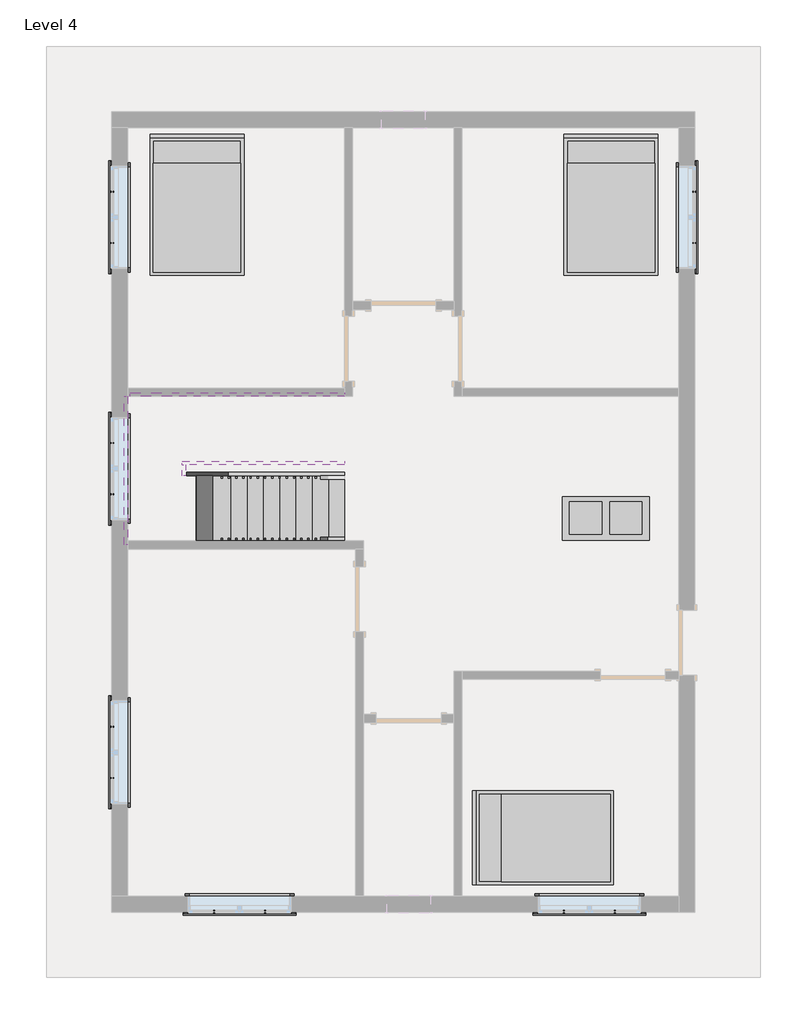
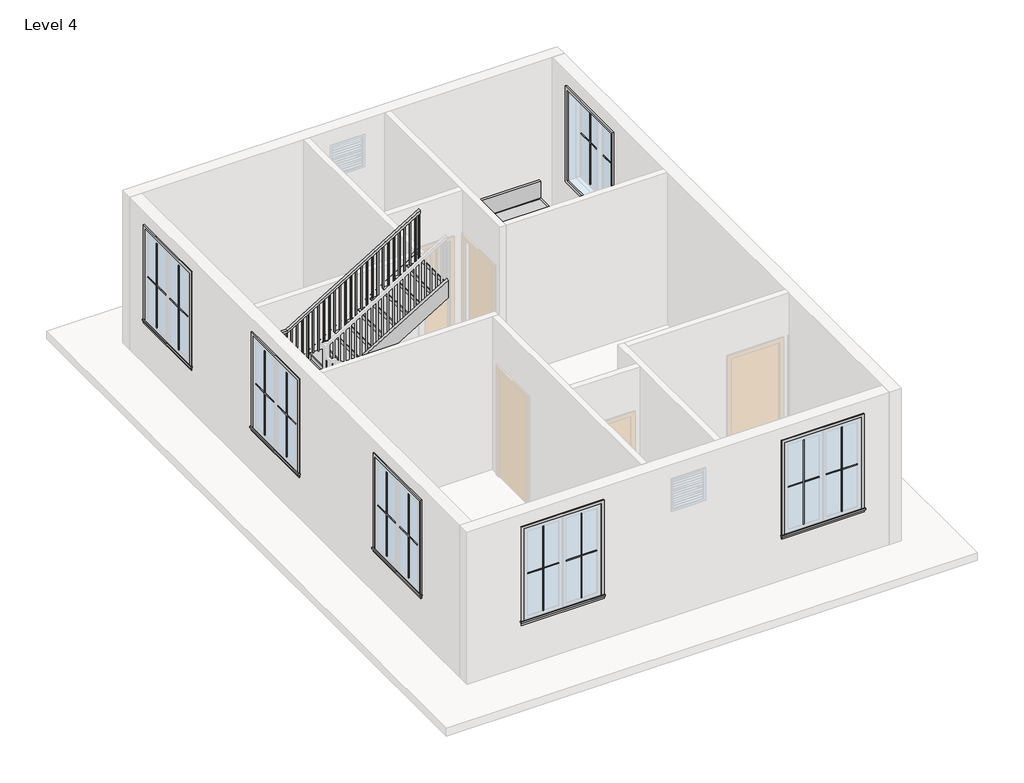
# One storey, part 2 of 2: 25 proxies, 6 members, 3 furniture elements, 1 railing, 1 stair flight.
"""IFC4 building model written with IfcOpenShell, lengths in millimetres."""

from ifc_helpers import new_model, si_unit, frame, origin, place, context, project, spatial, polyline, outline, extrude, faceted_brep, transform, mapped, element, save
from components import muntin_pattern_2x2_muntin_pattern_2x2_bff912c5, muntin_pattern_2x2_muntin_pattern_2x2_c2194282, trim_window_exterior_flat_with_sill_e04b3088, trim_window_interior_flat_picture_frame_2a7685fe, coffee_table_with_brass_mullions_11320_coffee_table_with_5962bef7, bed_17739_bed_17739_15c61121, stair_flight_94d610a2

model = new_model("IFC4")

# Units and contexts
model_context = context("Model", 3, world=origin())
ifc_project = project(units=[si_unit("LENGTHUNIT", "METRE", prefix="MILLI")], contexts=[model_context])

# Site, building, storey
site = spatial("IfcSite", under=ifc_project)
building = spatial("IfcBuilding", under=site)
storey = spatial("IfcBuildingStorey", under=building, Name="Level 4", Elevation=6400.8)

# Proxies
placement = place(None, origin())
muntin_pattern_2x2_muntin_pattern_2x2_shape = muntin_pattern_2x2_muntin_pattern_2x2_bff912c5(model_context)
element("IfcBuildingElementProxy", 1, Name="Muntin Pattern_2x2 : Muntin Pattern_2x2", ObjectType="Muntin Pattern_2x2 : Muntin Pattern_2x2", at=placement, inside=storey, context=model_context, shape_type="MappedRepresentation", body=[
    mapped(muntin_pattern_2x2_muntin_pattern_2x2_shape, transform((-3196.8535855, -5792.3946383, 7385.05), x_axis=(-1.0, 0.0, 0.0), y_axis=(0.0, -1.0, 0.0), z_axis=(0.0, 0.0, 1.0))),
])
element("IfcBuildingElementProxy", 2, Name="Muntin Pattern_2x2 : Muntin Pattern_2x2", ObjectType="Muntin Pattern_2x2 : Muntin Pattern_2x2", at=placement, inside=storey, context=model_context, shape_type="MappedRepresentation", body=[
    mapped(muntin_pattern_2x2_muntin_pattern_2x2_shape, transform((-5347.9160855, -3914.3821383, 7385.05), x_axis=(0.0, 1.0, 0.0), y_axis=(-1.0, 0.0, 0.0), z_axis=(0.0, 0.0, 1.0))),
])
element("IfcBuildingElementProxy", 3, Name="Muntin Pattern_2x2 : Muntin Pattern_2x2", ObjectType="Muntin Pattern_2x2 : Muntin Pattern_2x2", at=placement, inside=storey, context=model_context, shape_type="MappedRepresentation", body=[
    mapped(muntin_pattern_2x2_muntin_pattern_2x2_shape, transform((1721.2214145, -5792.3946383, 7385.05), x_axis=(-1.0, 0.0, 0.0), y_axis=(0.0, -1.0, 0.0), z_axis=(0.0, 0.0, 1.0))),
])
element("IfcBuildingElementProxy", 4, Name="Muntin Pattern_2x2 : Muntin Pattern_2x2", ObjectType="Muntin Pattern_2x2 : Muntin Pattern_2x2", at=placement, inside=storey, context=model_context, shape_type="MappedRepresentation", body=[
    mapped(muntin_pattern_2x2_muntin_pattern_2x2_shape, transform((2837.2339145, 4324.7428617, 7385.05), x_axis=(0.0, -1.0, 0.0), y_axis=(1.0, 0.0, 0.0), z_axis=(0.0, 0.0, 1.0))),
])
element("IfcBuildingElementProxy", 5, Name="Muntin Pattern_2x2 : Muntin Pattern_2x2", ObjectType="Muntin Pattern_2x2 : Muntin Pattern_2x2", at=placement, inside=storey, context=model_context, shape_type="MappedRepresentation", body=[
    mapped(muntin_pattern_2x2_muntin_pattern_2x2_shape, transform((-5347.9160855, 3604.0178617, 7385.05), x_axis=(0.0, 1.0, 0.0), y_axis=(-1.0, 0.0, 0.0), z_axis=(0.0, 0.0, 1.0))),
])
element("IfcBuildingElementProxy", 6, Name="Muntin Pattern_2x2 : Muntin Pattern_2x2", ObjectType="Muntin Pattern_2x2 : Muntin Pattern_2x2", at=placement, inside=storey, context=model_context, shape_type="MappedRepresentation", body=[
    mapped(muntin_pattern_2x2_muntin_pattern_2x2_shape, transform((-5347.9160855, 73.4178617, 7385.05), x_axis=(0.0, 1.0, 0.0), y_axis=(-1.0, 0.0, 0.0), z_axis=(0.0, 0.0, 1.0))),
])
muntin_pattern_2x2_muntin_pattern_2x2_2_shape = muntin_pattern_2x2_muntin_pattern_2x2_c2194282(model_context)
element("IfcBuildingElementProxy", 7, Name="Muntin Pattern_2x2 : Muntin Pattern_2x2", ObjectType="Muntin Pattern_2x2 : Muntin Pattern_2x2", at=placement, inside=storey, context=model_context, shape_type="MappedRepresentation", body=[
    mapped(muntin_pattern_2x2_muntin_pattern_2x2_2_shape, transform((-3917.5785855, -5792.3946383, 7385.05), x_axis=(1.0, 0.0, 0.0), y_axis=(0.0, 1.0, 0.0), z_axis=(0.0, 0.0, 1.0))),
])
element("IfcBuildingElementProxy", 8, Name="Muntin Pattern_2x2 : Muntin Pattern_2x2", ObjectType="Muntin Pattern_2x2 : Muntin Pattern_2x2", at=placement, inside=storey, context=model_context, shape_type="MappedRepresentation", body=[
    mapped(muntin_pattern_2x2_muntin_pattern_2x2_2_shape, transform((-5347.9160855, -3193.6571383, 7385.05), x_axis=(0.0, -1.0, 0.0), y_axis=(1.0, 0.0, 0.0), z_axis=(0.0, 0.0, 1.0))),
])
element("IfcBuildingElementProxy", 9, Name="Muntin Pattern_2x2 : Muntin Pattern_2x2", ObjectType="Muntin Pattern_2x2 : Muntin Pattern_2x2", at=placement, inside=storey, context=model_context, shape_type="MappedRepresentation", body=[
    mapped(muntin_pattern_2x2_muntin_pattern_2x2_2_shape, transform((1000.4964145, -5792.3946383, 7385.05), x_axis=(1.0, 0.0, 0.0), y_axis=(0.0, 1.0, 0.0), z_axis=(0.0, 0.0, 1.0))),
])
element("IfcBuildingElementProxy", 10, Name="Muntin Pattern_2x2 : Muntin Pattern_2x2", ObjectType="Muntin Pattern_2x2 : Muntin Pattern_2x2", at=placement, inside=storey, context=model_context, shape_type="MappedRepresentation", body=[
    mapped(muntin_pattern_2x2_muntin_pattern_2x2_2_shape, transform((2837.2339145, 3604.0178617, 7385.05), x_axis=(0.0, 1.0, 0.0), y_axis=(-1.0, 0.0, 0.0), z_axis=(0.0, 0.0, 1.0))),
])
element("IfcBuildingElementProxy", 11, Name="Muntin Pattern_2x2 : Muntin Pattern_2x2", ObjectType="Muntin Pattern_2x2 : Muntin Pattern_2x2", at=placement, inside=storey, context=model_context, shape_type="MappedRepresentation", body=[
    mapped(muntin_pattern_2x2_muntin_pattern_2x2_2_shape, transform((-5347.9160855, 4324.7428617, 7385.05), x_axis=(0.0, -1.0, 0.0), y_axis=(1.0, 0.0, 0.0), z_axis=(0.0, 0.0, 1.0))),
])
element("IfcBuildingElementProxy", 12, Name="Muntin Pattern_2x2 : Muntin Pattern_2x2", ObjectType="Muntin Pattern_2x2 : Muntin Pattern_2x2", at=placement, inside=storey, context=model_context, shape_type="MappedRepresentation", body=[
    mapped(muntin_pattern_2x2_muntin_pattern_2x2_2_shape, transform((-5347.9160855, 794.1428617, 7385.05), x_axis=(0.0, -1.0, 0.0), y_axis=(1.0, 0.0, 0.0), z_axis=(0.0, 0.0, 1.0))),
])
trim_window_exterior_flat_with_sill_shape = trim_window_exterior_flat_with_sill_e04b3088(model_context)
element("IfcBuildingElementProxy", 13, Name="Trim-Window-Exterior-Flat : with Sill", ObjectType="Trim-Window-Exterior-Flat : with Sill", at=placement, inside=storey, context=model_context, shape_type="MappedRepresentation", body=[
    mapped(trim_window_exterior_flat_with_sill_shape, transform((-3557.2160855, -5801.9196383, 9144.0), x_axis=(1.0, 0.0, 0.0), y_axis=(0.0, 0.0, 1.0), z_axis=(0.0, -1.0, 0.0))),
])
element("IfcBuildingElementProxy", 14, Name="Trim-Window-Exterior-Flat : with Sill", ObjectType="Trim-Window-Exterior-Flat : with Sill", at=placement, inside=storey, context=model_context, shape_type="MappedRepresentation", body=[
    mapped(trim_window_exterior_flat_with_sill_shape, transform((-5357.4410855, -3554.0196383, 9144.0), x_axis=(0.0, -1.0, 0.0), y_axis=(0.0, 0.0, 1.0), z_axis=(-1.0, 0.0, 0.0))),
])
element("IfcBuildingElementProxy", 15, Name="Trim-Window-Exterior-Flat : with Sill", ObjectType="Trim-Window-Exterior-Flat : with Sill", at=placement, inside=storey, context=model_context, shape_type="MappedRepresentation", body=[
    mapped(trim_window_exterior_flat_with_sill_shape, transform((1360.8589145, -5801.9196383, 9144.0), x_axis=(1.0, 0.0, 0.0), y_axis=(0.0, 0.0, 1.0), z_axis=(0.0, -1.0, 0.0))),
])
element("IfcBuildingElementProxy", 16, Name="Trim-Window-Exterior-Flat : with Sill", ObjectType="Trim-Window-Exterior-Flat : with Sill", at=placement, inside=storey, context=model_context, shape_type="MappedRepresentation", body=[
    mapped(trim_window_exterior_flat_with_sill_shape, transform((2846.7589145, 3964.3803617, 9144.0), x_axis=(0.0, 1.0, 0.0), y_axis=(0.0, 0.0, 1.0), z_axis=(1.0, 0.0, 0.0))),
])
element("IfcBuildingElementProxy", 17, Name="Trim-Window-Exterior-Flat : with Sill", ObjectType="Trim-Window-Exterior-Flat : with Sill", at=placement, inside=storey, context=model_context, shape_type="MappedRepresentation", body=[
    mapped(trim_window_exterior_flat_with_sill_shape, transform((-5357.4410855, 3964.3803617, 9144.0), x_axis=(0.0, -1.0, 0.0), y_axis=(0.0, 0.0, 1.0), z_axis=(-1.0, 0.0, 0.0))),
])
element("IfcBuildingElementProxy", 18, Name="Trim-Window-Exterior-Flat : with Sill", ObjectType="Trim-Window-Exterior-Flat : with Sill", at=placement, inside=storey, context=model_context, shape_type="MappedRepresentation", body=[
    mapped(trim_window_exterior_flat_with_sill_shape, transform((-5357.4410855, 433.7803617, 9144.0), x_axis=(0.0, -1.0, 0.0), y_axis=(0.0, 0.0, 1.0), z_axis=(-1.0, 0.0, 0.0))),
])
trim_window_interior_flat_picture_frame_shape = trim_window_interior_flat_picture_frame_2a7685fe(model_context)
element("IfcBuildingElementProxy", 19, Name="Trim-Window-Interior-Flat : Picture Frame", ObjectType="Trim-Window-Interior-Flat : Picture Frame", at=placement, inside=storey, context=model_context, shape_type="MappedRepresentation", body=[
    mapped(trim_window_interior_flat_picture_frame_shape, transform((-3557.2160855, -5573.3196383, 9144.0), x_axis=(-1.0, 0.0, 0.0), y_axis=(0.0, 0.0, 1.0), z_axis=(0.0, 1.0, 0.0))),
])
element("IfcBuildingElementProxy", 20, Name="Trim-Window-Interior-Flat : Picture Frame", ObjectType="Trim-Window-Interior-Flat : Picture Frame", at=placement, inside=storey, context=model_context, shape_type="MappedRepresentation", body=[
    mapped(trim_window_interior_flat_picture_frame_shape, transform((-5128.8410855, -3554.0196383, 9144.0), x_axis=(0.0, 1.0, 0.0), y_axis=(0.0, 0.0, 1.0), z_axis=(1.0, 0.0, 0.0))),
])
element("IfcBuildingElementProxy", 21, Name="Trim-Window-Interior-Flat : Picture Frame", ObjectType="Trim-Window-Interior-Flat : Picture Frame", at=placement, inside=storey, context=model_context, shape_type="MappedRepresentation", body=[
    mapped(trim_window_interior_flat_picture_frame_shape, transform((1360.8589145, -5573.3196383, 9144.0), x_axis=(-1.0, 0.0, 0.0), y_axis=(0.0, 0.0, 1.0), z_axis=(0.0, 1.0, 0.0))),
])
element("IfcBuildingElementProxy", 22, Name="Trim-Window-Interior-Flat : Picture Frame", ObjectType="Trim-Window-Interior-Flat : Picture Frame", at=placement, inside=storey, context=model_context, shape_type="MappedRepresentation", body=[
    mapped(trim_window_interior_flat_picture_frame_shape, transform((2618.1589145, 3964.3803617, 9144.0), x_axis=(0.0, -1.0, 0.0), y_axis=(0.0, 0.0, 1.0), z_axis=(-1.0, 0.0, 0.0))),
])
element("IfcBuildingElementProxy", 23, Name="Trim-Window-Interior-Flat : Picture Frame", ObjectType="Trim-Window-Interior-Flat : Picture Frame", at=placement, inside=storey, context=model_context, shape_type="MappedRepresentation", body=[
    mapped(trim_window_interior_flat_picture_frame_shape, transform((-5128.8410855, 3964.3803617, 9144.0), x_axis=(0.0, 1.0, 0.0), y_axis=(0.0, 0.0, 1.0), z_axis=(1.0, 0.0, 0.0))),
])
element("IfcBuildingElementProxy", 24, Name="Trim-Window-Interior-Flat : Picture Frame", ObjectType="Trim-Window-Interior-Flat : Picture Frame", at=placement, inside=storey, context=model_context, shape_type="MappedRepresentation", body=[
    mapped(trim_window_interior_flat_picture_frame_shape, transform((-5128.8410855, 433.7803617, 9144.0), x_axis=(0.0, 1.0, 0.0), y_axis=(0.0, 0.0, 1.0), z_axis=(1.0, 0.0, 0.0))),
])
coffee_table_with_brass_mullions_11320_coffee_table_with_shape = coffee_table_with_brass_mullions_11320_coffee_table_with_5962bef7(model_context)
element("IfcBuildingElementProxy", 25, Name="coffee_table_with_brass_mullions_11320 : coffee_table_with_brass_mullions_11320", ObjectType="coffee_table_with_brass_mullions_11320 : coffee_table_with_brass_mullions_11320", at=placement, inside=storey, context=model_context, shape_type="MappedRepresentation", body=[
    mapped(coffee_table_with_brass_mullions_11320_coffee_table_with_shape, transform((2229.2258874, -696.5196383, 6400.8), x_axis=(1.0, 0.0, 0.0), y_axis=(0.0, 1.0, 0.0), z_axis=(0.0, 0.0, 1.0))),
])

# Furniture
bed_17739_bed_17739_shape = bed_17739_bed_17739_15c61121(model_context)
element("IfcFurniture", 26, ObjectType="Bed_17739 : Bed_17739", at=placement, inside=storey, context=model_context, shape_type="MappedRepresentation", body=[
    mapped(bed_17739_bed_17739_shape, transform((1665.6589145, 4116.7803617, 6400.8), x_axis=(1.0, 0.0, 0.0), y_axis=(0.0, 1.0, 0.0), z_axis=(0.0, 0.0, 1.0))),
])
element("IfcFurniture", 27, ObjectType="Bed_17739 : Bed_17739", at=placement, inside=storey, context=model_context, shape_type="MappedRepresentation", body=[
    mapped(bed_17739_bed_17739_shape, transform((-4157.2910855, 4116.7803617, 6400.8), x_axis=(1.0, 0.0, 0.0), y_axis=(0.0, 1.0, 0.0), z_axis=(0.0, 0.0, 1.0))),
])
element("IfcFurniture", 28, ObjectType="Bed_17739 : Bed_17739", at=placement, inside=storey, context=model_context, shape_type="MappedRepresentation", body=[
    mapped(bed_17739_bed_17739_shape, transform((732.2089145, -4754.5725945, 6400.8), x_axis=(0.0, 1.0, 0.0), y_axis=(-1.0, 0.0, 0.0), z_axis=(0.0, 0.0, 1.0))),
])

# Members
element("IfcMember", 29, ObjectType="Stringer - 2\" Width", at=placement, inside=storey, context=model_context, shape_type="SweptSolid", body=[
    extrude(outline(polyline([(6400.8, -2080.8410855), (6612.914512, -2080.8410855), (8001.0, -4371.1821407), (8001.0, -4959.2565972), (6400.8, -2318.9265972), (6400.8, -2080.8410855)])), frame((0.0, -633.0196383, 0.0), z_axis=(0.0, 1.0, 0.0), x_axis=(0.0, 0.0, 1.0)), (0.0, 0.0, 1.0), 50.8),
])
element("IfcMember", 30, ObjectType="Stringer - 2\" Width", at=placement, inside=storey, context=model_context, shape_type="SweptSolid", body=[
    extrude(outline(polyline([(-5128.8410855, -633.0196383), (-5179.6410855, -633.0196383), (-5179.6410855, 1449.7803617), (-5128.8410855, 1449.7803617), (-5128.8410855, -633.0196383)])), frame((0.0, 0.0, 7696.2), z_axis=(0.0, 0.0, 1.0), x_axis=(1.0, 0.0, 0.0)), (0.0, 0.0, 1.0), 304.8),
])
element("IfcMember", 31, ObjectType="Stringer - 2\" Width", at=placement, inside=storey, context=model_context, shape_type="SweptSolid", body=[
    extrude(outline(polyline([(7696.2, -4505.9455737), (9165.9602959, -2080.8410855), (9522.3690574, -2080.8410855), (7696.2, -5094.0200302), (7696.2, -4505.9455737)])), frame((0.0, 1449.7803617, 0.0), z_axis=(0.0, 1.0, 0.0), x_axis=(0.0, 0.0, 1.0)), (0.0, 0.0, 1.0), 50.8),
])
element("IfcMember", 32, ObjectType="Stringer - 2\" Width", at=placement, inside=storey, context=model_context, shape_type="SweptSolid", body=[
    extrude(outline(polyline([(6400.8, -2080.8410855), (6612.914512, -2080.8410855), (7967.5811786, -4316.0410855), (7611.1724171, -4316.0410855), (6400.8, -2318.9265972), (6400.8, -2080.8410855)])), frame((0.0, 332.1803617, 0.0), z_axis=(0.0, 1.0, 0.0), x_axis=(0.0, 0.0, 1.0)), (0.0, 0.0, 1.0), 50.8),
])
element("IfcMember", 33, ObjectType="Stringer - 2\" Width", at=placement, inside=storey, context=model_context, shape_type="SweptSolid", body=[
    extrude(outline(polyline([(-4316.0410855, 332.1803617), (-4366.8410855, 332.1803617), (-4366.8410855, 484.5803617), (-4316.0410855, 484.5803617), (-4316.0410855, 332.1803617)])), frame((0.0, 0.0, 7696.2), z_axis=(0.0, 0.0, 1.0), x_axis=(1.0, 0.0, 0.0)), (0.0, 0.0, 1.0), 304.8),
])
element("IfcMember", 34, ObjectType="Stringer - 2\" Width", at=placement, inside=storey, context=model_context, shape_type="SweptSolid", body=[
    extrude(outline(polyline([(8136.914512, -4366.8410855), (7780.5057504, -4366.8410855), (9165.9602959, -2080.8410855), (9522.3690574, -2080.8410855), (8136.914512, -4366.8410855)])), frame((0.0, 484.5803617, 0.0), z_axis=(0.0, 1.0, 0.0), x_axis=(0.0, 0.0, 1.0)), (0.0, 0.0, 1.0), 50.8),
])

# Railing
element("IfcRailing", 35, ObjectType="Handrail - Rectangular", at=placement, inside=storey, context=model_context, shape_type="SolidModel", body=[
    faceted_brep([(-2080.8410855, -582.2196383, 7453.7454545), (-2080.8410855, -582.2196383, 7394.3439943), (-2080.8410855, -531.4196383, 7394.3439943), (-2080.8410855, -531.4196383, 7453.7454545), (-4366.8410855, -582.2196383, 8839.2), (-4381.0334949, -582.2196383, 8788.4), (-4381.0334949, -531.4196383, 8788.4), (-4366.8410855, -531.4196383, 8839.2), (-5128.8410855, -582.2196383, 8839.2), (-5128.8410855, -582.2196383, 8788.4), (-5078.0410855, -531.4196383, 8788.4), (-5078.0410855, -531.4196383, 8839.2), (-5128.8410855, 1449.7803617, 8839.2), (-5128.8410855, 1449.7803617, 8788.4), (-5078.0410855, 1398.9803617, 8788.4), (-5078.0410855, 1398.9803617, 8839.2), (-4595.4410855, 1449.7803617, 8839.2), (-4581.2486761, 1449.7803617, 8788.4), (-4581.2486761, 1398.9803617, 8788.4), (-4595.4410855, 1398.9803617, 8839.2), (-2080.8410855, 1449.7803617, 10363.2), (-2080.8410855, 1398.9803617, 10363.2), (-2080.8410855, 1398.9803617, 10303.7985397), (-2080.8410855, 1449.7803617, 10303.7985397)], [[[0, 1, 2, 3]], [[1, 0, 4, 5]], [[2, 1, 5, 6]], [[3, 2, 6, 7]], [[0, 3, 7, 4]], [[5, 4, 8, 9]], [[6, 5, 9, 10]], [[7, 6, 10, 11]], [[4, 7, 11, 8]], [[9, 8, 12, 13]], [[10, 9, 13, 14]], [[11, 10, 14, 15]], [[8, 11, 15, 12]], [[13, 12, 16, 17]], [[14, 13, 17, 18]], [[15, 14, 18, 19]], [[12, 15, 19, 16]], [[20, 21, 22, 23]], [[17, 16, 20, 23]], [[18, 17, 23, 22]], [[19, 18, 22, 21]], [[16, 19, 21, 20]]]),
    extrude(outline(polyline([(10251.8439943, -2166.5660855), (9310.2545455, -2166.5660855), (9310.2545455, -2147.5160855), (10263.3894488, -2147.5160855), (10251.8439943, -2166.5660855)])), frame((0.0, 1414.8553617, 0.0), z_axis=(0.0, 1.0, 0.0), x_axis=(0.0, 0.0, 1.0)), (0.0, 0.0, 1.0), 19.05),
    extrude(outline(polyline([(10190.2682367, -2268.1660855), (9310.2545455, -2268.1660855), (9310.2545455, -2249.1160855), (10201.8136913, -2249.1160855), (10190.2682367, -2268.1660855)])), frame((0.0, 1414.8553617, 0.0), z_axis=(0.0, 1.0, 0.0), x_axis=(0.0, 0.0, 1.0)), (0.0, 0.0, 1.0), 19.05),
    extrude(outline(polyline([(10128.6924791, -2369.7660855), (9171.7090909, -2369.7660855), (9171.7090909, -2350.7160855), (10140.2379337, -2350.7160855), (10128.6924791, -2369.7660855)])), frame((0.0, 1414.8553617, 0.0), z_axis=(0.0, 1.0, 0.0), x_axis=(0.0, 0.0, 1.0)), (0.0, 0.0, 1.0), 19.05),
    extrude(outline(polyline([(10067.1167216, -2471.3660855), (9171.7090909, -2471.3660855), (9171.7090909, -2452.3160855), (10078.6621761, -2452.3160855), (10067.1167216, -2471.3660855)])), frame((0.0, 1414.8553617, 0.0), z_axis=(0.0, 1.0, 0.0), x_axis=(0.0, 0.0, 1.0)), (0.0, 0.0, 1.0), 19.05),
    extrude(outline(polyline([(10005.540964, -2572.9660855), (9033.1636364, -2572.9660855), (9033.1636364, -2553.9160855), (10017.0864185, -2553.9160855), (10005.540964, -2572.9660855)])), frame((0.0, 1414.8553617, 0.0), z_axis=(0.0, 1.0, 0.0), x_axis=(0.0, 0.0, 1.0)), (0.0, 0.0, 1.0), 19.05),
    extrude(outline(polyline([(9943.9652064, -2674.5660855), (9033.1636364, -2674.5660855), (9033.1636364, -2655.5160855), (9955.510661, -2655.5160855), (9943.9652064, -2674.5660855)])), frame((0.0, 1414.8553617, 0.0), z_axis=(0.0, 1.0, 0.0), x_axis=(0.0, 0.0, 1.0)), (0.0, 0.0, 1.0), 19.05),
    extrude(outline(polyline([(9882.3894488, -2776.1660855), (9033.1636364, -2776.1660855), (9033.1636364, -2757.1160855), (9893.9349034, -2757.1160855), (9882.3894488, -2776.1660855)])), frame((0.0, 1414.8553617, 0.0), z_axis=(0.0, 1.0, 0.0), x_axis=(0.0, 0.0, 1.0)), (0.0, 0.0, 1.0), 19.05),
    extrude(outline(polyline([(9820.8136913, -2877.7660855), (8894.6181818, -2877.7660855), (8894.6181818, -2858.7160855), (9832.3591458, -2858.7160855), (9820.8136913, -2877.7660855)])), frame((0.0, 1414.8553617, 0.0), z_axis=(0.0, 1.0, 0.0), x_axis=(0.0, 0.0, 1.0)), (0.0, 0.0, 1.0), 19.05),
    extrude(outline(polyline([(9759.2379337, -2979.3660855), (8894.6181818, -2979.3660855), (8894.6181818, -2960.3160855), (9770.7833882, -2960.3160855), (9759.2379337, -2979.3660855)])), frame((0.0, 1414.8553617, 0.0), z_axis=(0.0, 1.0, 0.0), x_axis=(0.0, 0.0, 1.0)), (0.0, 0.0, 1.0), 19.05),
    extrude(outline(polyline([(9697.6621761, -3080.9660855), (8756.0727273, -3080.9660855), (8756.0727273, -3061.9160855), (9709.2076307, -3061.9160855), (9697.6621761, -3080.9660855)])), frame((0.0, 1414.8553617, 0.0), z_axis=(0.0, 1.0, 0.0), x_axis=(0.0, 0.0, 1.0)), (0.0, 0.0, 1.0), 19.05),
    extrude(outline(polyline([(9636.0864185, -3182.5660855), (8756.0727273, -3182.5660855), (8756.0727273, -3163.5160855), (9647.6318731, -3163.5160855), (9636.0864185, -3182.5660855)])), frame((0.0, 1414.8553617, 0.0), z_axis=(0.0, 1.0, 0.0), x_axis=(0.0, 0.0, 1.0)), (0.0, 0.0, 1.0), 19.05),
    extrude(outline(polyline([(9574.510661, -3284.1660855), (8617.5272727, -3284.1660855), (8617.5272727, -3265.1160855), (9586.0561155, -3265.1160855), (9574.510661, -3284.1660855)])), frame((0.0, 1414.8553617, 0.0), z_axis=(0.0, 1.0, 0.0), x_axis=(0.0, 0.0, 1.0)), (0.0, 0.0, 1.0), 19.05),
    extrude(outline(polyline([(9512.9349034, -3385.7660855), (8617.5272727, -3385.7660855), (8617.5272727, -3366.7160855), (9524.4803579, -3366.7160855), (9512.9349034, -3385.7660855)])), frame((0.0, 1414.8553617, 0.0), z_axis=(0.0, 1.0, 0.0), x_axis=(0.0, 0.0, 1.0)), (0.0, 0.0, 1.0), 19.05),
    extrude(outline(polyline([(9451.3591458, -3487.3660855), (8478.9818182, -3487.3660855), (8478.9818182, -3468.3160855), (9462.9046004, -3468.3160855), (9451.3591458, -3487.3660855)])), frame((0.0, 1414.8553617, 0.0), z_axis=(0.0, 1.0, 0.0), x_axis=(0.0, 0.0, 1.0)), (0.0, 0.0, 1.0), 19.05),
    extrude(outline(polyline([(9389.7833882, -3588.9660855), (8478.9818182, -3588.9660855), (8478.9818182, -3569.9160855), (9401.3288428, -3569.9160855), (9389.7833882, -3588.9660855)])), frame((0.0, 1414.8553617, 0.0), z_axis=(0.0, 1.0, 0.0), x_axis=(0.0, 0.0, 1.0)), (0.0, 0.0, 1.0), 19.05),
    extrude(outline(polyline([(9328.2076307, -3690.5660855), (8478.9818182, -3690.5660855), (8478.9818182, -3671.5160855), (9339.7530852, -3671.5160855), (9328.2076307, -3690.5660855)])), frame((0.0, 1414.8553617, 0.0), z_axis=(0.0, 1.0, 0.0), x_axis=(0.0, 0.0, 1.0)), (0.0, 0.0, 1.0), 19.05),
    extrude(outline(polyline([(9266.6318731, -3792.1660855), (8340.4363636, -3792.1660855), (8340.4363636, -3773.1160855), (9278.1773276, -3773.1160855), (9266.6318731, -3792.1660855)])), frame((0.0, 1414.8553617, 0.0), z_axis=(0.0, 1.0, 0.0), x_axis=(0.0, 0.0, 1.0)), (0.0, 0.0, 1.0), 19.05),
    extrude(outline(polyline([(9205.0561155, -3893.7660855), (8340.4363636, -3893.7660855), (8340.4363636, -3874.7160855), (9216.60157, -3874.7160855), (9205.0561155, -3893.7660855)])), frame((0.0, 1414.8553617, 0.0), z_axis=(0.0, 1.0, 0.0), x_axis=(0.0, 0.0, 1.0)), (0.0, 0.0, 1.0), 19.05),
    extrude(outline(polyline([(9143.4803579, -3995.3660855), (8201.8909091, -3995.3660855), (8201.8909091, -3976.3160855), (9155.0258125, -3976.3160855), (9143.4803579, -3995.3660855)])), frame((0.0, 1414.8553617, 0.0), z_axis=(0.0, 1.0, 0.0), x_axis=(0.0, 0.0, 1.0)), (0.0, 0.0, 1.0), 19.05),
    extrude(outline(polyline([(9081.9046004, -4096.9660855), (8201.8909091, -4096.9660855), (8201.8909091, -4077.9160855), (9093.4500549, -4077.9160855), (9081.9046004, -4096.9660855)])), frame((0.0, 1414.8553617, 0.0), z_axis=(0.0, 1.0, 0.0), x_axis=(0.0, 0.0, 1.0)), (0.0, 0.0, 1.0), 19.05),
    extrude(outline(polyline([(9020.3288428, -4198.5660855), (8063.3454545, -4198.5660855), (8063.3454545, -4179.5160855), (9031.8742973, -4179.5160855), (9020.3288428, -4198.5660855)])), frame((0.0, 1414.8553617, 0.0), z_axis=(0.0, 1.0, 0.0), x_axis=(0.0, 0.0, 1.0)), (0.0, 0.0, 1.0), 19.05),
    extrude(outline(polyline([(8958.7530852, -4300.1660855), (8063.3454545, -4300.1660855), (8063.3454545, -4281.1160855), (8970.2985397, -4281.1160855), (8958.7530852, -4300.1660855)])), frame((0.0, 1414.8553617, 0.0), z_axis=(0.0, 1.0, 0.0), x_axis=(0.0, 0.0, 1.0)), (0.0, 0.0, 1.0), 19.05),
    extrude(outline(polyline([(8897.1773276, -4401.7660855), (7924.8, -4401.7660855), (7924.8, -4382.7160855), (8908.7227822, -4382.7160855), (8897.1773276, -4401.7660855)])), frame((0.0, 1414.8553617, 0.0), z_axis=(0.0, 1.0, 0.0), x_axis=(0.0, 0.0, 1.0)), (0.0, 0.0, 1.0), 19.05),
    extrude(outline(polyline([(8835.60157, -4503.3660855), (7924.8, -4503.3660855), (7924.8, -4484.3160855), (8847.1470246, -4484.3160855), (8835.60157, -4503.3660855)])), frame((0.0, 1414.8553617, 0.0), z_axis=(0.0, 1.0, 0.0), x_axis=(0.0, 0.0, 1.0)), (0.0, 0.0, 1.0), 19.05),
    extrude(outline(polyline([(-4604.9660855, 1433.9053617), (-4585.9160855, 1433.9053617), (-4585.9160855, 1414.8553617), (-4604.9660855, 1414.8553617), (-4604.9660855, 1433.9053617)])), frame((0.0, 0.0, 7924.8), z_axis=(0.0, 0.0, 1.0), x_axis=(1.0, 0.0, 0.0)), (0.0, 0.0, 1.0), 863.6),
    extrude(outline(polyline([(-4706.5660855, 1433.9053617), (-4687.5160855, 1433.9053617), (-4687.5160855, 1414.8553617), (-4706.5660855, 1414.8553617), (-4706.5660855, 1433.9053617)])), frame((0.0, 0.0, 7924.8), z_axis=(0.0, 0.0, 1.0), x_axis=(1.0, 0.0, 0.0)), (0.0, 0.0, 1.0), 863.6),
    extrude(outline(polyline([(-4808.1660855, 1433.9053617), (-4789.1160855, 1433.9053617), (-4789.1160855, 1414.8553617), (-4808.1660855, 1414.8553617), (-4808.1660855, 1433.9053617)])), frame((0.0, 0.0, 7924.8), z_axis=(0.0, 0.0, 1.0), x_axis=(1.0, 0.0, 0.0)), (0.0, 0.0, 1.0), 863.6),
    extrude(outline(polyline([(-4909.7660855, 1433.9053617), (-4890.7160855, 1433.9053617), (-4890.7160855, 1414.8553617), (-4909.7660855, 1414.8553617), (-4909.7660855, 1433.9053617)])), frame((0.0, 0.0, 7924.8), z_axis=(0.0, 0.0, 1.0), x_axis=(1.0, 0.0, 0.0)), (0.0, 0.0, 1.0), 863.6),
    extrude(outline(polyline([(-5011.3660855, 1433.9053617), (-4992.3160855, 1433.9053617), (-4992.3160855, 1414.8553617), (-5011.3660855, 1414.8553617), (-5011.3660855, 1433.9053617)])), frame((0.0, 0.0, 7924.8), z_axis=(0.0, 0.0, 1.0), x_axis=(1.0, 0.0, 0.0)), (0.0, 0.0, 1.0), 863.6),
    extrude(outline(polyline([(-5112.9660855, 1364.0553617), (-5112.9660855, 1383.1053617), (-5093.9160855, 1383.1053617), (-5093.9160855, 1364.0553617), (-5112.9660855, 1364.0553617)])), frame((0.0, 0.0, 7924.8), z_axis=(0.0, 0.0, 1.0), x_axis=(1.0, 0.0, 0.0)), (0.0, 0.0, 1.0), 863.6),
    extrude(outline(polyline([(-5112.9660855, 1262.4553617), (-5112.9660855, 1281.5053617), (-5093.9160855, 1281.5053617), (-5093.9160855, 1262.4553617), (-5112.9660855, 1262.4553617)])), frame((0.0, 0.0, 7924.8), z_axis=(0.0, 0.0, 1.0), x_axis=(1.0, 0.0, 0.0)), (0.0, 0.0, 1.0), 863.6),
    extrude(outline(polyline([(-5112.9660855, 1160.8553617), (-5112.9660855, 1179.9053617), (-5093.9160855, 1179.9053617), (-5093.9160855, 1160.8553617), (-5112.9660855, 1160.8553617)])), frame((0.0, 0.0, 7924.8), z_axis=(0.0, 0.0, 1.0), x_axis=(1.0, 0.0, 0.0)), (0.0, 0.0, 1.0), 863.6),
    extrude(outline(polyline([(-5112.9660855, 1059.2553617), (-5112.9660855, 1078.3053617), (-5093.9160855, 1078.3053617), (-5093.9160855, 1059.2553617), (-5112.9660855, 1059.2553617)])), frame((0.0, 0.0, 7924.8), z_axis=(0.0, 0.0, 1.0), x_axis=(1.0, 0.0, 0.0)), (0.0, 0.0, 1.0), 863.6),
    extrude(outline(polyline([(-5112.9660855, 957.6553617), (-5112.9660855, 976.7053617), (-5093.9160855, 976.7053617), (-5093.9160855, 957.6553617), (-5112.9660855, 957.6553617)])), frame((0.0, 0.0, 7924.8), z_axis=(0.0, 0.0, 1.0), x_axis=(1.0, 0.0, 0.0)), (0.0, 0.0, 1.0), 863.6),
    extrude(outline(polyline([(-5112.9660855, 856.0553617), (-5112.9660855, 875.1053617), (-5093.9160855, 875.1053617), (-5093.9160855, 856.0553617), (-5112.9660855, 856.0553617)])), frame((0.0, 0.0, 7924.8), z_axis=(0.0, 0.0, 1.0), x_axis=(1.0, 0.0, 0.0)), (0.0, 0.0, 1.0), 863.6),
    extrude(outline(polyline([(-5112.9660855, 754.4553617), (-5112.9660855, 773.5053617), (-5093.9160855, 773.5053617), (-5093.9160855, 754.4553617), (-5112.9660855, 754.4553617)])), frame((0.0, 0.0, 7924.8), z_axis=(0.0, 0.0, 1.0), x_axis=(1.0, 0.0, 0.0)), (0.0, 0.0, 1.0), 863.6),
    extrude(outline(polyline([(-5112.9660855, 652.8553617), (-5112.9660855, 671.9053617), (-5093.9160855, 671.9053617), (-5093.9160855, 652.8553617), (-5112.9660855, 652.8553617)])), frame((0.0, 0.0, 7924.8), z_axis=(0.0, 0.0, 1.0), x_axis=(1.0, 0.0, 0.0)), (0.0, 0.0, 1.0), 863.6),
    extrude(outline(polyline([(-5112.9660855, 551.2553617), (-5112.9660855, 570.3053617), (-5093.9160855, 570.3053617), (-5093.9160855, 551.2553617), (-5112.9660855, 551.2553617)])), frame((0.0, 0.0, 7924.8), z_axis=(0.0, 0.0, 1.0), x_axis=(1.0, 0.0, 0.0)), (0.0, 0.0, 1.0), 863.6),
    extrude(outline(polyline([(-5112.9660855, 449.6553617), (-5112.9660855, 468.7053617), (-5093.9160855, 468.7053617), (-5093.9160855, 449.6553617), (-5112.9660855, 449.6553617)])), frame((0.0, 0.0, 7924.8), z_axis=(0.0, 0.0, 1.0), x_axis=(1.0, 0.0, 0.0)), (0.0, 0.0, 1.0), 863.6),
    extrude(outline(polyline([(-5112.9660855, 348.0553617), (-5112.9660855, 367.1053617), (-5093.9160855, 367.1053617), (-5093.9160855, 348.0553617), (-5112.9660855, 348.0553617)])), frame((0.0, 0.0, 7924.8), z_axis=(0.0, 0.0, 1.0), x_axis=(1.0, 0.0, 0.0)), (0.0, 0.0, 1.0), 863.6),
    extrude(outline(polyline([(-5112.9660855, 246.4553617), (-5112.9660855, 265.5053617), (-5093.9160855, 265.5053617), (-5093.9160855, 246.4553617), (-5112.9660855, 246.4553617)])), frame((0.0, 0.0, 7924.8), z_axis=(0.0, 0.0, 1.0), x_axis=(1.0, 0.0, 0.0)), (0.0, 0.0, 1.0), 863.6),
    extrude(outline(polyline([(-5112.9660855, 144.8553617), (-5112.9660855, 163.9053617), (-5093.9160855, 163.9053617), (-5093.9160855, 144.8553617), (-5112.9660855, 144.8553617)])), frame((0.0, 0.0, 7924.8), z_axis=(0.0, 0.0, 1.0), x_axis=(1.0, 0.0, 0.0)), (0.0, 0.0, 1.0), 863.6),
    extrude(outline(polyline([(-5112.9660855, 43.2553617), (-5112.9660855, 62.3053617), (-5093.9160855, 62.3053617), (-5093.9160855, 43.2553617), (-5112.9660855, 43.2553617)])), frame((0.0, 0.0, 7924.8), z_axis=(0.0, 0.0, 1.0), x_axis=(1.0, 0.0, 0.0)), (0.0, 0.0, 1.0), 863.6),
    extrude(outline(polyline([(-5112.9660855, -58.3446383), (-5112.9660855, -39.2946383), (-5093.9160855, -39.2946383), (-5093.9160855, -58.3446383), (-5112.9660855, -58.3446383)])), frame((0.0, 0.0, 7924.8), z_axis=(0.0, 0.0, 1.0), x_axis=(1.0, 0.0, 0.0)), (0.0, 0.0, 1.0), 863.6),
    extrude(outline(polyline([(-5112.9660855, -159.9446383), (-5112.9660855, -140.8946383), (-5093.9160855, -140.8946383), (-5093.9160855, -159.9446383), (-5112.9660855, -159.9446383)])), frame((0.0, 0.0, 7924.8), z_axis=(0.0, 0.0, 1.0), x_axis=(1.0, 0.0, 0.0)), (0.0, 0.0, 1.0), 863.6),
    extrude(outline(polyline([(-5112.9660855, -261.5446383), (-5112.9660855, -242.4946383), (-5093.9160855, -242.4946383), (-5093.9160855, -261.5446383), (-5112.9660855, -261.5446383)])), frame((0.0, 0.0, 7924.8), z_axis=(0.0, 0.0, 1.0), x_axis=(1.0, 0.0, 0.0)), (0.0, 0.0, 1.0), 863.6),
    extrude(outline(polyline([(-5112.9660855, -363.1446383), (-5112.9660855, -344.0946383), (-5093.9160855, -344.0946383), (-5093.9160855, -363.1446383), (-5112.9660855, -363.1446383)])), frame((0.0, 0.0, 7924.8), z_axis=(0.0, 0.0, 1.0), x_axis=(1.0, 0.0, 0.0)), (0.0, 0.0, 1.0), 863.6),
    extrude(outline(polyline([(-5112.9660855, -464.7446383), (-5112.9660855, -445.6946383), (-5093.9160855, -445.6946383), (-5093.9160855, -464.7446383), (-5112.9660855, -464.7446383)])), frame((0.0, 0.0, 7924.8), z_axis=(0.0, 0.0, 1.0), x_axis=(1.0, 0.0, 0.0)), (0.0, 0.0, 1.0), 863.6),
    extrude(outline(polyline([(-5017.7160855, -566.3446383), (-5036.7660855, -566.3446383), (-5036.7660855, -547.2946383), (-5017.7160855, -547.2946383), (-5017.7160855, -566.3446383)])), frame((0.0, 0.0, 7924.8), z_axis=(0.0, 0.0, 1.0), x_axis=(1.0, 0.0, 0.0)), (0.0, 0.0, 1.0), 863.6),
    extrude(outline(polyline([(-4916.1160855, -566.3446383), (-4935.1660855, -566.3446383), (-4935.1660855, -547.2946383), (-4916.1160855, -547.2946383), (-4916.1160855, -566.3446383)])), frame((0.0, 0.0, 7924.8), z_axis=(0.0, 0.0, 1.0), x_axis=(1.0, 0.0, 0.0)), (0.0, 0.0, 1.0), 863.6),
    extrude(outline(polyline([(-4814.5160855, -566.3446383), (-4833.5660855, -566.3446383), (-4833.5660855, -547.2946383), (-4814.5160855, -547.2946383), (-4814.5160855, -566.3446383)])), frame((0.0, 0.0, 7924.8), z_axis=(0.0, 0.0, 1.0), x_axis=(1.0, 0.0, 0.0)), (0.0, 0.0, 1.0), 863.6),
    extrude(outline(polyline([(-4712.9160855, -566.3446383), (-4731.9660855, -566.3446383), (-4731.9660855, -547.2946383), (-4712.9160855, -547.2946383), (-4712.9160855, -566.3446383)])), frame((0.0, 0.0, 7924.8), z_axis=(0.0, 0.0, 1.0), x_axis=(1.0, 0.0, 0.0)), (0.0, 0.0, 1.0), 863.6),
    extrude(outline(polyline([(-4611.3160855, -566.3446383), (-4630.3660855, -566.3446383), (-4630.3660855, -547.2946383), (-4611.3160855, -547.2946383), (-4611.3160855, -566.3446383)])), frame((0.0, 0.0, 7924.8), z_axis=(0.0, 0.0, 1.0), x_axis=(1.0, 0.0, 0.0)), (0.0, 0.0, 1.0), 863.6),
    extrude(outline(polyline([(-4509.7160855, -566.3446383), (-4528.7660855, -566.3446383), (-4528.7660855, -547.2946383), (-4509.7160855, -547.2946383), (-4509.7160855, -566.3446383)])), frame((0.0, 0.0, 7924.8), z_axis=(0.0, 0.0, 1.0), x_axis=(1.0, 0.0, 0.0)), (0.0, 0.0, 1.0), 863.6),
    extrude(outline(polyline([(-4408.1160855, -566.3446383), (-4427.1660855, -566.3446383), (-4427.1660855, -547.2946383), (-4408.1160855, -547.2946383), (-4408.1160855, -566.3446383)])), frame((0.0, 0.0, 7924.8), z_axis=(0.0, 0.0, 1.0), x_axis=(1.0, 0.0, 0.0)), (0.0, 0.0, 1.0), 863.6),
    extrude(outline(polyline([(8754.7833882, -4325.5660855), (7786.2545455, -4325.5660855), (7786.2545455, -4306.5160855), (8743.2379337, -4306.5160855), (8754.7833882, -4325.5660855)])), frame((0.0, -566.3446383, 0.0), z_axis=(0.0, 1.0, 0.0), x_axis=(0.0, 0.0, 1.0)), (0.0, 0.0, 1.0), 19.05),
    extrude(outline(polyline([(8693.2076307, -4223.9660855), (7786.2545455, -4223.9660855), (7786.2545455, -4204.9160855), (8681.6621761, -4204.9160855), (8693.2076307, -4223.9660855)])), frame((0.0, -566.3446383, 0.0), z_axis=(0.0, 1.0, 0.0), x_axis=(0.0, 0.0, 1.0)), (0.0, 0.0, 1.0), 19.05),
    extrude(outline(polyline([(8631.6318731, -4122.3660855), (7647.7090909, -4122.3660855), (7647.7090909, -4103.3160855), (8620.0864185, -4103.3160855), (8631.6318731, -4122.3660855)])), frame((0.0, -566.3446383, 0.0), z_axis=(0.0, 1.0, 0.0), x_axis=(0.0, 0.0, 1.0)), (0.0, 0.0, 1.0), 19.05),
    extrude(outline(polyline([(8570.0561155, -4020.7660855), (7647.7090909, -4020.7660855), (7647.7090909, -4001.7160855), (8558.510661, -4001.7160855), (8570.0561155, -4020.7660855)])), frame((0.0, -566.3446383, 0.0), z_axis=(0.0, 1.0, 0.0), x_axis=(0.0, 0.0, 1.0)), (0.0, 0.0, 1.0), 19.05),
    extrude(outline(polyline([(8508.4803579, -3919.1660855), (7647.7090909, -3919.1660855), (7647.7090909, -3900.1160855), (8496.9349034, -3900.1160855), (8508.4803579, -3919.1660855)])), frame((0.0, -566.3446383, 0.0), z_axis=(0.0, 1.0, 0.0), x_axis=(0.0, 0.0, 1.0)), (0.0, 0.0, 1.0), 19.05),
    extrude(outline(polyline([(8446.9046004, -3817.5660855), (7509.1636364, -3817.5660855), (7509.1636364, -3798.5160855), (8435.3591458, -3798.5160855), (8446.9046004, -3817.5660855)])), frame((0.0, -566.3446383, 0.0), z_axis=(0.0, 1.0, 0.0), x_axis=(0.0, 0.0, 1.0)), (0.0, 0.0, 1.0), 19.05),
    extrude(outline(polyline([(8385.3288428, -3715.9660855), (7509.1636364, -3715.9660855), (7509.1636364, -3696.9160855), (8373.7833882, -3696.9160855), (8385.3288428, -3715.9660855)])), frame((0.0, -566.3446383, 0.0), z_axis=(0.0, 1.0, 0.0), x_axis=(0.0, 0.0, 1.0)), (0.0, 0.0, 1.0), 19.05),
    extrude(outline(polyline([(8323.7530852, -3614.3660855), (7370.6181818, -3614.3660855), (7370.6181818, -3595.3160855), (8312.2076307, -3595.3160855), (8323.7530852, -3614.3660855)])), frame((0.0, -566.3446383, 0.0), z_axis=(0.0, 1.0, 0.0), x_axis=(0.0, 0.0, 1.0)), (0.0, 0.0, 1.0), 19.05),
    extrude(outline(polyline([(8262.1773276, -3512.7660855), (7370.6181818, -3512.7660855), (7370.6181818, -3493.7160855), (8250.6318731, -3493.7160855), (8262.1773276, -3512.7660855)])), frame((0.0, -566.3446383, 0.0), z_axis=(0.0, 1.0, 0.0), x_axis=(0.0, 0.0, 1.0)), (0.0, 0.0, 1.0), 19.05),
    extrude(outline(polyline([(8200.60157, -3411.1660855), (7232.0727273, -3411.1660855), (7232.0727273, -3392.1160855), (8189.0561155, -3392.1160855), (8200.60157, -3411.1660855)])), frame((0.0, -566.3446383, 0.0), z_axis=(0.0, 1.0, 0.0), x_axis=(0.0, 0.0, 1.0)), (0.0, 0.0, 1.0), 19.05),
    extrude(outline(polyline([(8139.0258125, -3309.5660855), (7232.0727273, -3309.5660855), (7232.0727273, -3290.5160855), (8127.4803579, -3290.5160855), (8139.0258125, -3309.5660855)])), frame((0.0, -566.3446383, 0.0), z_axis=(0.0, 1.0, 0.0), x_axis=(0.0, 0.0, 1.0)), (0.0, 0.0, 1.0), 19.05),
    extrude(outline(polyline([(8077.4500549, -3207.9660855), (7093.5272727, -3207.9660855), (7093.5272727, -3188.9160855), (8065.9046004, -3188.9160855), (8077.4500549, -3207.9660855)])), frame((0.0, -566.3446383, 0.0), z_axis=(0.0, 1.0, 0.0), x_axis=(0.0, 0.0, 1.0)), (0.0, 0.0, 1.0), 19.05),
    extrude(outline(polyline([(8015.8742973, -3106.3660855), (7093.5272727, -3106.3660855), (7093.5272727, -3087.3160855), (8004.3288428, -3087.3160855), (8015.8742973, -3106.3660855)])), frame((0.0, -566.3446383, 0.0), z_axis=(0.0, 1.0, 0.0), x_axis=(0.0, 0.0, 1.0)), (0.0, 0.0, 1.0), 19.05),
    extrude(outline(polyline([(7954.2985397, -3004.7660855), (7093.5272727, -3004.7660855), (7093.5272727, -2985.7160855), (7942.7530852, -2985.7160855), (7954.2985397, -3004.7660855)])), frame((0.0, -566.3446383, 0.0), z_axis=(0.0, 1.0, 0.0), x_axis=(0.0, 0.0, 1.0)), (0.0, 0.0, 1.0), 19.05),
    extrude(outline(polyline([(7892.7227822, -2903.1660855), (6954.9818182, -2903.1660855), (6954.9818182, -2884.1160855), (7881.1773276, -2884.1160855), (7892.7227822, -2903.1660855)])), frame((0.0, -566.3446383, 0.0), z_axis=(0.0, 1.0, 0.0), x_axis=(0.0, 0.0, 1.0)), (0.0, 0.0, 1.0), 19.05),
    extrude(outline(polyline([(7831.1470246, -2801.5660855), (6954.9818182, -2801.5660855), (6954.9818182, -2782.5160855), (7819.60157, -2782.5160855), (7831.1470246, -2801.5660855)])), frame((0.0, -566.3446383, 0.0), z_axis=(0.0, 1.0, 0.0), x_axis=(0.0, 0.0, 1.0)), (0.0, 0.0, 1.0), 19.05),
    extrude(outline(polyline([(7769.571267, -2699.9660855), (6816.4363636, -2699.9660855), (6816.4363636, -2680.9160855), (7758.0258125, -2680.9160855), (7769.571267, -2699.9660855)])), frame((0.0, -566.3446383, 0.0), z_axis=(0.0, 1.0, 0.0), x_axis=(0.0, 0.0, 1.0)), (0.0, 0.0, 1.0), 19.05),
    extrude(outline(polyline([(7707.9955094, -2598.3660855), (6816.4363636, -2598.3660855), (6816.4363636, -2579.3160855), (7696.4500549, -2579.3160855), (7707.9955094, -2598.3660855)])), frame((0.0, -566.3446383, 0.0), z_axis=(0.0, 1.0, 0.0), x_axis=(0.0, 0.0, 1.0)), (0.0, 0.0, 1.0), 19.05),
    extrude(outline(polyline([(7646.4197519, -2496.7660855), (6677.8909091, -2496.7660855), (6677.8909091, -2477.7160855), (7634.8742973, -2477.7160855), (7646.4197519, -2496.7660855)])), frame((0.0, -566.3446383, 0.0), z_axis=(0.0, 1.0, 0.0), x_axis=(0.0, 0.0, 1.0)), (0.0, 0.0, 1.0), 19.05),
    extrude(outline(polyline([(7584.8439943, -2395.1660855), (6677.8909091, -2395.1660855), (6677.8909091, -2376.1160855), (7573.2985397, -2376.1160855), (7584.8439943, -2395.1660855)])), frame((0.0, -566.3446383, 0.0), z_axis=(0.0, 1.0, 0.0), x_axis=(0.0, 0.0, 1.0)), (0.0, 0.0, 1.0), 19.05),
    extrude(outline(polyline([(7523.2682367, -2293.5660855), (6539.3454545, -2293.5660855), (6539.3454545, -2274.5160855), (7511.7227822, -2274.5160855), (7523.2682367, -2293.5660855)])), frame((0.0, -566.3446383, 0.0), z_axis=(0.0, 1.0, 0.0), x_axis=(0.0, 0.0, 1.0)), (0.0, 0.0, 1.0), 19.05),
    extrude(outline(polyline([(7461.6924791, -2191.9660855), (6539.3454545, -2191.9660855), (6539.3454545, -2172.9160855), (7450.1470246, -2172.9160855), (7461.6924791, -2191.9660855)])), frame((0.0, -566.3446383, 0.0), z_axis=(0.0, 1.0, 0.0), x_axis=(0.0, 0.0, 1.0)), (0.0, 0.0, 1.0), 19.05),
    extrude(outline(polyline([(-5112.9660855, 1414.8553617), (-5112.9660855, 1433.9053617), (-5093.9160855, 1433.9053617), (-5093.9160855, 1414.8553617), (-5112.9660855, 1414.8553617)])), frame((0.0, 0.0, 7924.8), z_axis=(0.0, 0.0, 1.0), x_axis=(1.0, 0.0, 0.0)), (0.0, 0.0, 1.0), 863.6),
    extrude(outline(polyline([(-5093.9160855, -566.3446383), (-5112.9660855, -566.3446383), (-5112.9660855, -547.2946383), (-5093.9160855, -547.2946383), (-5093.9160855, -566.3446383)])), frame((0.0, 0.0, 7924.8), z_axis=(0.0, 0.0, 1.0), x_axis=(1.0, 0.0, 0.0)), (0.0, 0.0, 1.0), 863.6),
    extrude(outline(polyline([(10292.2530852, -2099.8910855), (9310.2545455, -2099.8910855), (9310.2545455, -2080.8410855), (10303.7985397, -2080.8410855), (10292.2530852, -2099.8910855)])), frame((0.0, 1414.8553617, 0.0), z_axis=(0.0, 1.0, 0.0), x_axis=(0.0, 0.0, 1.0)), (0.0, 0.0, 1.0), 19.05),
    extrude(outline(polyline([(7405.8894488, -2099.8910855), (6539.3454545, -2099.8910855), (6539.3454545, -2080.8410855), (7394.3439943, -2080.8410855), (7405.8894488, -2099.8910855)])), frame((0.0, -566.3446383, 0.0), z_axis=(0.0, 1.0, 0.0), x_axis=(0.0, 0.0, 1.0)), (0.0, 0.0, 1.0), 19.05),
])

# Stair flight
stair_flight_shape = stair_flight_94d610a2(model_context)
element("IfcStairFlight", 36, ObjectType="2\" Tread 1\" Nosing 1/4\" Riser", at=placement, inside=storey, context=model_context, shape_type="MappedRepresentation", body=[
    mapped(stair_flight_shape, transform((0.0, 0.0, 0.0), x_axis=(1.0, 0.0, 0.0), y_axis=(0.0, 1.0, 0.0), z_axis=(0.0, 0.0, 1.0))),
])

save(model, "model.ifc")

# Revit data of these elements
# Type "Muntin Pattern_2x2 : Muntin Pattern_2x2"
#   Width [instance default] = 4' - 0"
#   Thickness = 0' - 0 1/2"
#   Height [instance default] = 4' - 0"
#   Distance = 0' - 0 3/4"
#   Interior Material [instance default] = none
#   Exterior Material [instance default] = none
#   Default Elevation = 0
# Type "Trim-Window-Exterior-Flat : with Sill"
#   Trim Width = 0' - 2 1/4"
#   Trim Thickness_Picture Frame = 0' - 1 1/4"
#   Trim Thickness_with Sill = 0' - 0 3/4"
#   Sill Thickness = 0' - 1 1/4"
#   Opening Width [instance default] = 2' - 0"
#   Opening Height [instance default] = 3' - 0"
#   Default Elevation = 4' - 0"
#   Sill = yes
#   Picture Frame = no
#   Trim Material [instance default] = none
# Type "Trim-Window-Interior-Flat : Picture Frame"
#   Trim Thickness_Picture Frame = 0' - 1 1/4"
#   Trim Width = 0' - 2 1/4"
#   Trim Thickness_with Sill = 0' - 0 3/4"
#   Sill Thickness = 0' - 1 1/4"
#   Opening Width [instance default] = 2' - 0"
#   Opening Height [instance default] = 3' - 0"
#   Default Elevation = 4' - 0"
#   Sill = no
#   Picture Frame = yes
#   Trim Material [instance default] = none
# Type "coffee_table_with_brass_mullions_11320 : coffee_table_with_brass_mullions_11320"
#   Default Elevation = 0
# Type "Bed_17739 : Bed_17739"
#   Default Elevation = 0
# Type "Handrail - Rectangular"
#   Assembly Code = "C2010400"
#   built-in parameter 1008612 = 0.0416667 (stored number, unit not read)
#   built-in parameter 1008611 = 0.0416667 (stored number, unit not read)
#   built-in parameter 1008609 = 0.333333 (stored number, unit not read)
#   built-in parameter 1008604 = 0.166667 (stored number, unit not read)
#   built-in parameter 1008603 = 0.166667 (stored number, unit not read)
#   Railing Height = 3' - 0"
#   built-in parameter 1008630 = 2
#   built-in parameter 1008610 = 2
#   built-in parameter 1008618 = Baluster - Square : 3/4"
# Elements 1, 2, 3, 4, 5, 6, 7, 8, 9, 10, 11, 12 (IfcBuildingElementProxy, "Muntin Pattern_2x2 : Muntin Pattern_2x2")
#   Width = 1' - 11 1/8"
#   Height = 5' - 6 1/2"
#   Interior Material = Wood - Stained
#   Exterior Material = Clad - White
#   Phase Created = New Construction
#   Materials on its faces: "Clad - White", "Wood - Stained"
# Elements 13, 14, 15, 16, 17, 18 (IfcBuildingElementProxy, "Trim-Window-Exterior-Flat : with Sill")
#   Opening Width = 4' - 9"
#   Opening Height = 6' - 0"
#   Trim Material = Clad - White
#   Phase Created = New Construction
#   Materials on its faces: "Clad - White"
# Elements 19, 20, 21, 22, 23, 24 (IfcBuildingElementProxy, "Trim-Window-Interior-Flat : Picture Frame")
#   Opening Width = 4' - 9"
#   Opening Height = 6' - 0"
#   Trim Material = Wood - Stained
#   Phase Created = New Construction
#   Materials on its faces: "Wood - Stained"
# Element 25 (IfcBuildingElementProxy, "coffee_table_with_brass_mullions_11320 : coffee_table_with_brass_mullions_11320")
#   Phase Created = New Construction
#   Materials on its faces: "Default Wall", "TABLE", "Glass", "Default"
# Elements 26, 27, 28 (IfcFurniture, "Bed_17739 : Bed_17739")
#   Phase Created = New Construction
#   Materials on its faces: "legs", "sheets", "bed frame", "Blanket"
# Elements 29, 30, 31, 32, 33, 34 (IfcMember, "Stringer - 2\" Width")
#   Phase Created = New Construction
# Element 35 (IfcRailing, "Handrail - Rectangular")
#   Phase Created = New Construction
# Element 36 (IfcStairFlight, "2\" Tread 1\" Nosing 1/4\" Riser")
#   Phase Created = New Construction
# Materials
#   "Clad - White": class "Wood", colour RGB 242 242 238, transparency 0, Cost = 0
#   "Wood - Stained": class "Wood", colour RGB 224 178 126, transparency 0, Cost = 0
#   "Default Wall": colour RGB 128 128 128, transparency 0, Cost = 0
#   "TABLE": class "Generic", colour RGB 120 120 120, transparency 0, Cost = 0
#   "Glass": class "Glass", colour RGB 0 128 192, transparency 0.75, Description = "Soda Lime Glass", Cost = 0
#   "Default": colour RGB 127 127 127, transparency 0, Cost = 0
#   "legs": colour RGB 90 73 37, transparency 0, Cost = 0
#   "sheets": colour RGB 200 195 176, transparency 0, Cost = 0
#   "bed frame": colour RGB 90 73 37, transparency 0, Cost = 0
#   "Blanket": class "System", colour RGB 59 0 1, transparency 0, Cost = 0
